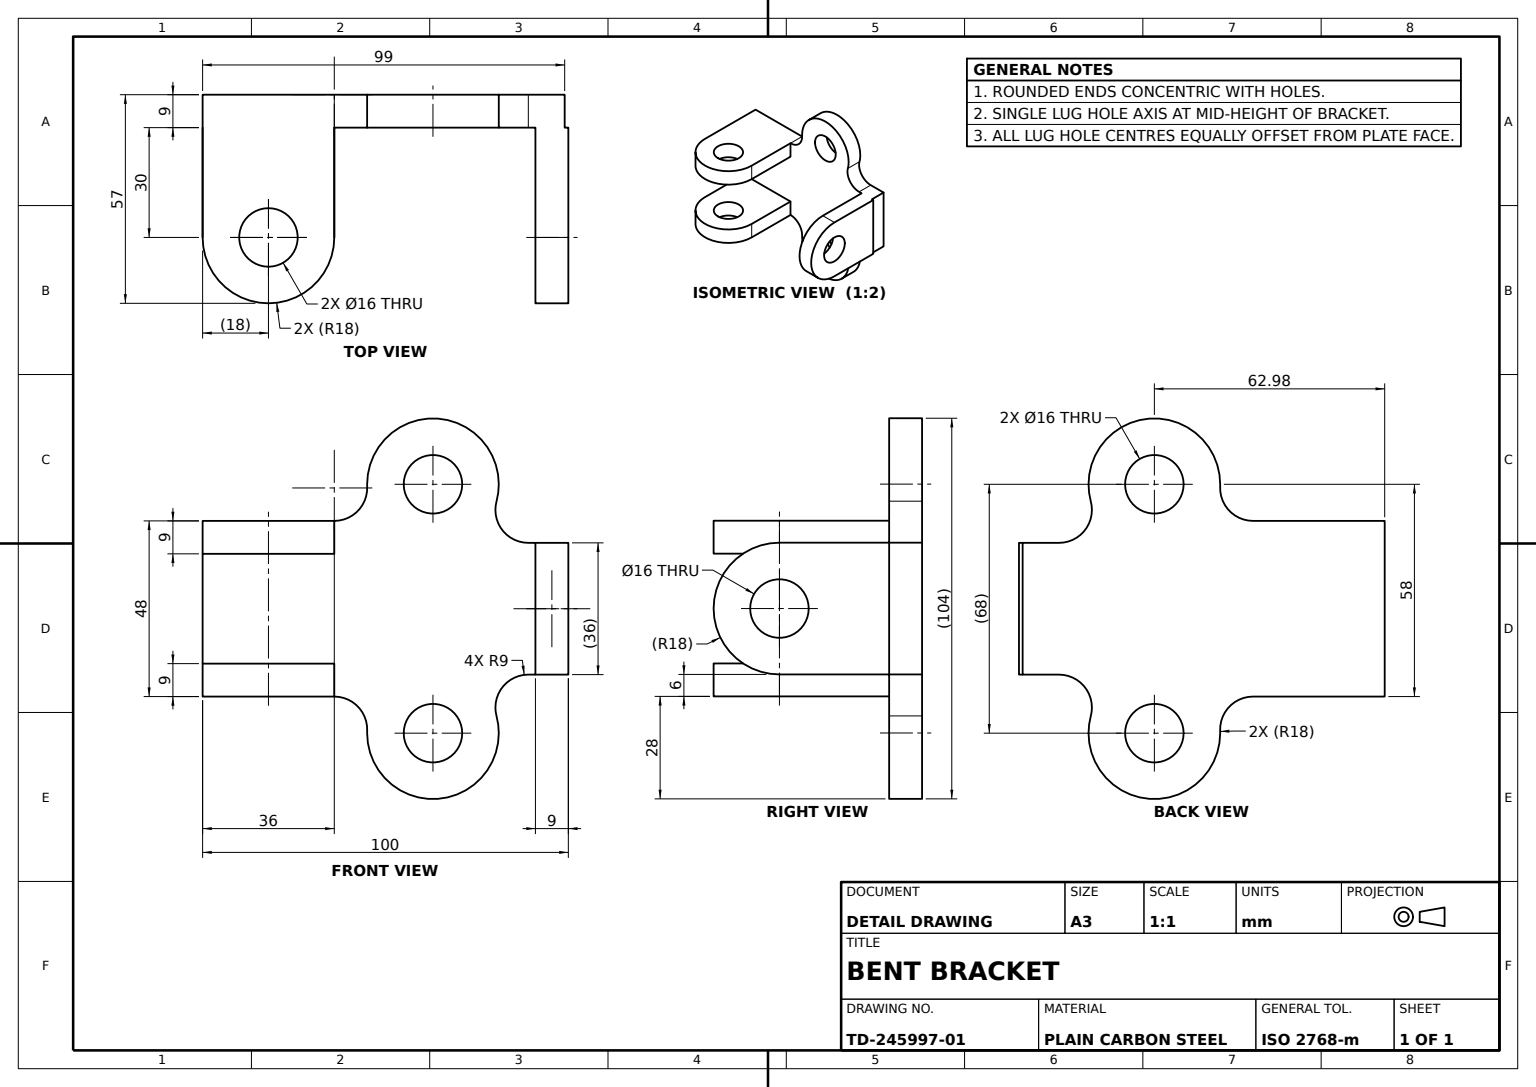
from build123d import *

# Parameters (mm, degrees)
BASE_PLATE_PROFILE_SKETCH_R = 8
BASE_PLATE_9MM_DEPTH        = 9
LUG_SKETCH_X100_R           = 8
LUG_X100_DEPTH              = 9
LUG_SKETCH_X0_R             = 8
LUG_X0_DEPTH                = 9
LUG_START                   = -9
LUG_SKETCH_OFFSET_48_R      = 8
LUG_OFFSET_48_DEPTH         = 9


with BuildPart() as part:
    # Base Plate Profile Sketch → Base Plate 9mm (new body)
    with BuildSketch(Plane.XY):
        with BuildLine():
            Line((0, 0), (0, 48))
            Line((0, 48), (36, 48))
            ThreePointArc((36, 48), (42.480740698, 50.755002002), (44.993825042, 57.333333333))
            ThreePointArc((44.993825042, 57.333333333), (65.004081247, 75.886001914), (80.366014874, 53.333333333))
            ThreePointArc((80.366014874, 53.333333333), (81.916856319, 45.522774425), (89.058284747, 42))
            Line((89.058284747, 42), (99, 42))
            Line((99, 42), (99, 24))
            Line((99, 24), (99, 6))
            Line((99, 6), (89.058284747, 6))
            ThreePointArc((89.058284747, 6), (81.916856319, 2.477225575), (80.366014874, -5.333333333))
            ThreePointArc((80.366014874, -5.333333333), (65.004081247, -27.886001914), (44.993825042, -9.333333333))
            ThreePointArc((44.993825042, -9.333333333), (42.480740698, -2.755002002), (36, 0))
            Line((36, 0), (0, 0))
        make_face()
        with Locations((62.981475126, 58)):
            Circle(BASE_PLATE_PROFILE_SKETCH_R, mode=Mode.SUBTRACT)
        with Locations((62.981475126, -10)):
            Circle(BASE_PLATE_PROFILE_SKETCH_R, mode=Mode.SUBTRACT)
    extrude(amount=BASE_PLATE_9MM_DEPTH)

    # Lug Sketch X100 → Lug X100 (add)
    with BuildSketch(Plane(origin=(100, 0, 0), x_dir=(0, 0, -1), z_dir=(1, 0, 0))):
        with BuildLine():
            Line((30, 42), (0, 42))
            Line((0, 42), (0, 6))
            Line((0, 6), (30, 6))
            ThreePointArc((30, 6), (48, 24), (30, 42))
        make_face()
        with Locations((30, 24)):
            Circle(LUG_SKETCH_X100_R, mode=Mode.SUBTRACT)
    extrude(amount=-LUG_X100_DEPTH)

    # Lug Sketch X0 → Lug X0 (add)
    with BuildSketch(Plane(origin=(0, 0, 0), x_dir=(1, 0, 0), z_dir=(0, 1, 0))):
        with BuildLine():
            Line((0, 30), (0, 0))
            Line((0, 0), (36, 0))
            Line((36, 0), (36, 30))
            ThreePointArc((36, 30), (18, 48), (0, 30))
        make_face()
        with Locations(Location((18, 30, 0), (0, 0, 270))):
            Circle(LUG_SKETCH_X0_R, mode=Mode.SUBTRACT)
    extrude(amount=LUG_X0_DEPTH)

    # Lug Sketch Offset 48 → Lug Offset 48 (add)
    with BuildSketch(Plane(origin=(0, 48, 0), x_dir=(1, 0, 0), z_dir=(0, 1, 0)).offset(LUG_START)):
        with BuildLine():
            Line((0, 30), (0, 0))
            Line((0, 0), (36, 0))
            Line((36, 0), (36, 30))
            ThreePointArc((36, 30), (18, 48), (0, 30))
        make_face()
        with Locations(Location((18, 30, 0), (0, 0, 270))):
            Circle(LUG_SKETCH_OFFSET_48_R, mode=Mode.SUBTRACT)
    extrude(amount=LUG_OFFSET_48_DEPTH)


solid = part.part
